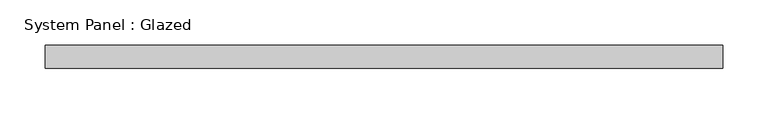
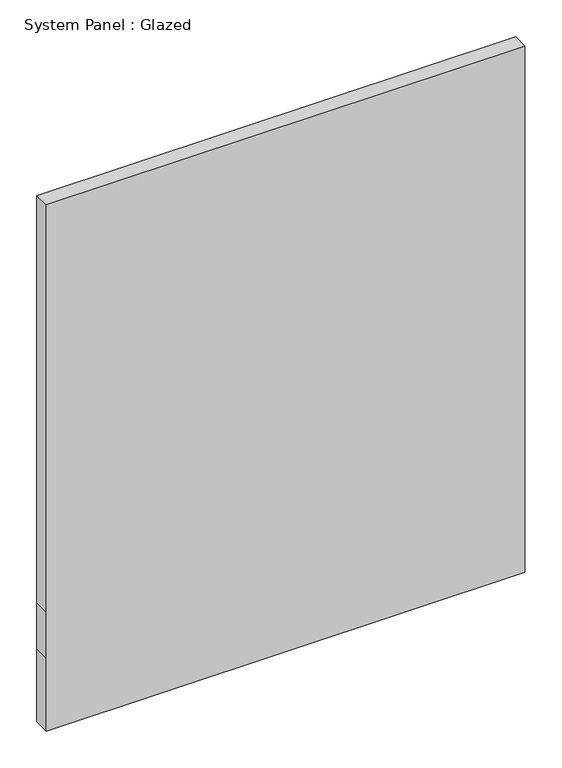
"""IFC4 building model written with IfcOpenShell, lengths in millimetres: plate geometry, System Panel : Glazed."""

from ifc_helpers import new_model, si_unit, frame, origin, place, context, project, spatial, polyline, outline, extrude, source, transform, mapped, element, save


def system_panel_glazed_a956e29f(model_context):
    return source(origin(), model_context, "Body", "SweptSolid", [
        extrude(outline(polyline([(0.0, -374.65), (0.0, 374.65), (120.65, 374.65), (196.85, 374.65), (869.95, 374.65), (869.95, -374.65), (196.85, -374.65), (120.65, -374.65), (0.0, -374.65)])), frame((0.0, 19.05, 0.0), z_axis=(0.0, 1.0, 0.0), x_axis=(0.0, 0.0, 1.0)), (0.0, 0.0, 1.0), 25.4),
    ])


if __name__ == "__main__":
    model = new_model("IFC4")
    model_context = context("Model", 3, world=origin())
    ifc_project = project(units=[si_unit("LENGTHUNIT", "METRE", prefix="MILLI")], contexts=[model_context])
    site = spatial("IfcSite", under=ifc_project)
    building = spatial("IfcBuilding", under=site)
    placement = place(None, origin())
    system_panel_glazed_shape = system_panel_glazed_a956e29f(model_context)
    element("IfcPlate", 1, ObjectType="System Panel : Glazed", at=placement, inside=building, context=model_context, shape_type="MappedRepresentation", body=[
        mapped(system_panel_glazed_shape, transform((0.0, 0.0, 0.0), x_axis=(1.0, 0.0, 0.0), y_axis=(0.0, 1.0, 0.0), z_axis=(0.0, 0.0, 1.0))),
    ])
    save(model, "model.ifc")

# Revit data of these elements
# Type "System Panel : Glazed"
#   Construction Type Id = "GSP4R"
#   Analytic Construction = "1/8 in Pilkington single glazing"
#   Visual Light Transmittance = 0.9
#   Solar Heat Gain Coefficient = 0.86
#   Heat Transfer Coefficient (U) = 1.18115 BTU/(h·ft²·°F)
#   Define Thermal Properties by = 1
# Element 1 (IfcPlate, "System Panel : Glazed")
#   Materials on its faces: "Glass"
# Materials
#   "Glass": class "Glass", colour RGB 0 128 192, transparency 0.75, Description = "Soda Lime Glass", Cost = 0
